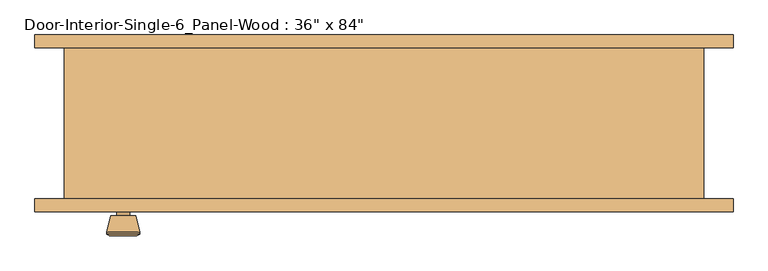
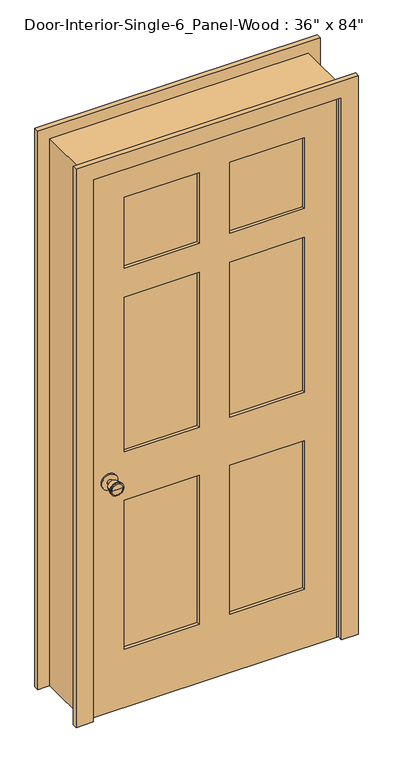
"""IFC4 building model written with IfcOpenShell, lengths in millimetres: door geometry."""

from ifc_helpers import new_model, si_unit, point, frame, frame_2d, origin, place, context, project, spatial, polyline, circle_curve, trimmed, segment, composite_curve, outline, extrude, faceted_brep, source, transform, mapped, element, save
from ifc_brep_helpers import plane_surface, cylinder_surface, revolved_surface, advanced_brep


def door_c5239341(model_context):
    return source(origin(), model_context, "Body", "SolidModel", [
        advanced_brep(
        [(-393.7, -70.2, 914.4), (-403.7, -70.2, 914.4), (-383.7, -70.2, 914.4), (-373.2241324, -21.2, 914.4), (-414.1758676, -21.2, 914.4), (-393.7, -21.2, 914.4), (-368.7, -23.0278681, 914.4), (-418.7, -23.0278681, 914.4), (-368.7, -26.4915463, 914.4), (-418.7, -26.4915463, 914.4), (-375.063764, -51.2, 914.4), (-412.336236, -51.2, 914.4), (-383.7, -51.2, 914.4), (-403.7, -51.2, 914.4)],
        [
            (0, 1),
            (1, 2, circle_curve(frame((-393.7, -70.2, 914.4), z_axis=(0.0, -1.0, 0.0), x_axis=(-1.0, 0.0, 0.0)), 10.0)),
            (2, 0),
            (2, 1, circle_curve(frame((-393.7, -70.2, 914.4), z_axis=(0.0, -1.0, 0.0), x_axis=(-1.0, 0.0, 0.0)), 10.0)),
            (3, 4, circle_curve(frame((-393.7, -21.2, 914.4), z_axis=(0.0, 1.0, 0.0), x_axis=(-1.0, 0.0, 0.0)), 20.4758676)),
            (4, 5),
            (5, 3),
            (4, 3, circle_curve(frame((-393.7, -21.2, 914.4), z_axis=(0.0, 1.0, 0.0), x_axis=(-1.0, 0.0, 0.0)), 20.4758676)),
            (6, 7, circle_curve(frame((-393.7, -23.0278681, 914.4), z_axis=(0.0, 1.0, 0.0), x_axis=(-1.0, 0.0, 0.0)), 25.0)),
            (7, 4),
            (3, 6),
            (7, 6, circle_curve(frame((-393.7, -23.0278681, 914.4), z_axis=(0.0, 1.0, 0.0), x_axis=(-1.0, 0.0, 0.0)), 25.0)),
            (8, 9, circle_curve(frame((-393.7, -26.4915463, 914.4), z_axis=(0.0, 1.0, 0.0), x_axis=(-1.0, 0.0, 0.0)), 25.0)),
            (9, 7),
            (6, 8),
            (9, 8, circle_curve(frame((-393.7, -26.4915463, 914.4), z_axis=(0.0, 1.0, 0.0), x_axis=(-1.0, 0.0, 0.0)), 25.0)),
            (10, 11, circle_curve(frame((-393.7, -51.2, 914.4), z_axis=(0.0, 1.0, 0.0), x_axis=(-1.0, 0.0, 0.0)), 18.636236)),
            (11, 9),
            (8, 10),
            (11, 10, circle_curve(frame((-393.7, -51.2, 914.4), z_axis=(0.0, 1.0, 0.0), x_axis=(-1.0, 0.0, 0.0)), 18.636236)),
            (12, 13, circle_curve(frame((-393.7, -51.2, 914.4), z_axis=(0.0, 1.0, 0.0), x_axis=(-1.0, 0.0, 0.0)), 10.0)),
            (13, 11),
            (10, 12),
            (13, 12, circle_curve(frame((-393.7, -51.2, 914.4), z_axis=(0.0, 1.0, 0.0), x_axis=(-1.0, 0.0, 0.0)), 10.0)),
            (1, 13),
            (12, 2),
        ],
        [
            plane_surface(frame((-393.7, -70.2, 914.4), z_axis=(0.0, -1.0, 0.0), x_axis=(-1.0, 0.0, 0.0))),
            plane_surface(frame((-393.7, -21.2, 914.4), z_axis=(0.0, 1.0, 0.0), x_axis=(-1.0, 0.0, 0.0))),
            revolved_surface(polyline([(-414.1758676, -21.2, 914.4), (-418.7, -23.0278681, 914.4)]), (-393.7, -70.2, 914.4), (0.0, -1.0, 0.0)),
            cylinder_surface(frame((-393.7, -70.2, 914.4), z_axis=(0.0, -1.0, 0.0), x_axis=(-1.0, 0.0, 0.0)), 25.0),
            revolved_surface(polyline([(-418.7, -26.4915463, 914.4), (-412.336236, -51.2, 914.4)]), (-393.7, -70.2, 914.4), (0.0, -1.0, 0.0)),
            plane_surface(frame((-393.7, -51.2, 914.4), z_axis=(0.0, -1.0, 0.0), x_axis=(-1.0, 0.0, 0.0))),
            cylinder_surface(frame((-393.7, -70.2, 914.4), z_axis=(0.0, -1.0, 0.0), x_axis=(-1.0, 0.0, 0.0)), 10.0),
        ],
        [
            (0, [[1, 2, 3]]),
            (0, [[-3, 4, -1]]),
            (1, [[5, 6, 7]]),
            (1, [[8, -7, -6]]),
            (2, [[9, 10, -5, 11]]),
            (2, [[12, -11, -8, -10]]),
            (3, [[13, 14, -9, 15]]),
            (3, [[16, -15, -12, -14]]),
            (4, [[17, 18, -13, 19]]),
            (4, [[20, -19, -16, -18]]),
            (5, [[21, 22, -17, 23]]),
            (5, [[24, -23, -20, -22]]),
            (6, [[-2, 25, -21, 26]]),
            (6, [[-4, -26, -24, -25]]),
        ],
    ),
        extrude(outline(composite_curve([segment(trimmed(circle_curve(frame_2d((914.4, -393.7)), 30.0), [point((914.4, -423.7))], [point((914.4, -363.7))], False, "CARTESIAN"), True, "CONTINUOUS"), segment(trimmed(circle_curve(frame_2d((914.4, -393.7)), 30.0), [point((914.4, -363.7))], [point((914.4, -423.7))], False, "CARTESIAN"), True, "CONTINUOUS")], self_intersect=False)), frame((0.0, -76.2, 0.0), z_axis=(0.0, 1.0, 0.0), x_axis=(0.0, 0.0, 1.0)), (0.0, 0.0, 1.0), 6.0),
        advanced_brep(
        [(-393.7, -117.125, 914.4), (-383.7, -117.125, 914.4), (-403.7, -117.125, 914.4), (-373.2241324, -166.125, 914.4), (-393.7, -166.125, 914.4), (-414.1758676, -166.125, 914.4), (-368.7, -164.2971319, 914.4), (-418.7, -164.2971319, 914.4), (-368.7, -160.8334537, 914.4), (-418.7, -160.8334537, 914.4), (-375.063764, -136.125, 914.4), (-412.336236, -136.125, 914.4), (-383.7, -136.125, 914.4), (-403.7, -136.125, 914.4)],
        [
            (0, 1),
            (1, 2, circle_curve(frame((-393.7, -117.125, 914.4), z_axis=(0.0, 1.0, 0.0), x_axis=(-1.0, 0.0, 0.0)), 10.0)),
            (2, 0),
            (2, 1, circle_curve(frame((-393.7, -117.125, 914.4), z_axis=(0.0, 1.0, 0.0), x_axis=(-1.0, 0.0, 0.0)), 10.0)),
            (3, 4),
            (4, 5),
            (5, 3, circle_curve(frame((-393.7, -166.125, 914.4), z_axis=(0.0, -1.0, 0.0), x_axis=(-1.0, 0.0, 0.0)), 20.4758676)),
            (3, 5, circle_curve(frame((-393.7, -166.125, 914.4), z_axis=(0.0, -1.0, 0.0), x_axis=(-1.0, 0.0, 0.0)), 20.4758676)),
            (6, 3),
            (5, 7),
            (7, 6, circle_curve(frame((-393.7, -164.2971319, 914.4), z_axis=(0.0, -1.0, 0.0), x_axis=(-1.0, 0.0, 0.0)), 25.0)),
            (6, 7, circle_curve(frame((-393.7, -164.2971319, 914.4), z_axis=(0.0, -1.0, 0.0), x_axis=(-1.0, 0.0, 0.0)), 25.0)),
            (8, 6),
            (7, 9),
            (9, 8, circle_curve(frame((-393.7, -160.8334537, 914.4), z_axis=(0.0, -1.0, 0.0), x_axis=(-1.0, 0.0, 0.0)), 25.0)),
            (8, 9, circle_curve(frame((-393.7, -160.8334537, 914.4), z_axis=(0.0, -1.0, 0.0), x_axis=(-1.0, 0.0, 0.0)), 25.0)),
            (10, 8),
            (9, 11),
            (11, 10, circle_curve(frame((-393.7, -136.125, 914.4), z_axis=(0.0, -1.0, 0.0), x_axis=(-1.0, 0.0, 0.0)), 18.636236)),
            (10, 11, circle_curve(frame((-393.7, -136.125, 914.4), z_axis=(0.0, -1.0, 0.0), x_axis=(-1.0, 0.0, 0.0)), 18.636236)),
            (12, 10),
            (11, 13),
            (13, 12, circle_curve(frame((-393.7, -136.125, 914.4), z_axis=(0.0, -1.0, 0.0), x_axis=(-1.0, 0.0, 0.0)), 10.0)),
            (12, 13, circle_curve(frame((-393.7, -136.125, 914.4), z_axis=(0.0, -1.0, 0.0), x_axis=(-1.0, 0.0, 0.0)), 10.0)),
            (1, 12),
            (13, 2),
        ],
        [
            plane_surface(frame((-393.7, -117.125, 914.4), z_axis=(0.0, 1.0, 0.0), x_axis=(-1.0, 0.0, 0.0))),
            plane_surface(frame((-393.7, -166.125, 914.4), z_axis=(0.0, -1.0, 0.0), x_axis=(-1.0, 0.0, 0.0))),
            revolved_surface(polyline([(-414.1758676, -166.125, 914.4), (-418.7, -164.2971319, 914.4)]), (-393.7, -117.125, 914.4), (0.0, 1.0, 0.0)),
            cylinder_surface(frame((-393.7, -117.125, 914.4), z_axis=(0.0, 1.0, 0.0), x_axis=(-1.0, 0.0, 0.0)), 25.0),
            revolved_surface(polyline([(-418.7, -160.8334537, 914.4), (-412.336236, -136.125, 914.4)]), (-393.7, -117.125, 914.4), (0.0, 1.0, 0.0)),
            plane_surface(frame((-393.7, -136.125, 914.4), z_axis=(0.0, 1.0, 0.0), x_axis=(-1.0, 0.0, 0.0))),
            cylinder_surface(frame((-393.7, -117.125, 914.4), z_axis=(0.0, 1.0, 0.0), x_axis=(-1.0, 0.0, 0.0)), 10.0),
        ],
        [
            (0, [[1, 2, 3]]),
            (0, [[-3, 4, -1]]),
            (1, [[5, 6, 7]]),
            (1, [[-6, -5, 8]]),
            (2, [[9, -7, 10, 11]]),
            (2, [[-10, -8, -9, 12]]),
            (3, [[13, -11, 14, 15]]),
            (3, [[-14, -12, -13, 16]]),
            (4, [[17, -15, 18, 19]]),
            (4, [[-18, -16, -17, 20]]),
            (5, [[21, -19, 22, 23]]),
            (5, [[-22, -20, -21, 24]]),
            (6, [[25, -23, 26, -2]]),
            (6, [[-26, -24, -25, -4]]),
        ],
    ),
        extrude(outline(composite_curve([segment(trimmed(circle_curve(frame_2d((914.4, -393.7)), 30.0), [point((914.4, -423.7))], [point((914.4, -363.7))], False, "CARTESIAN"), True, "CONTINUOUS"), segment(trimmed(circle_curve(frame_2d((914.4, -393.7)), 30.0), [point((914.4, -363.7))], [point((914.4, -423.7))], False, "CARTESIAN"), True, "CONTINUOUS")], self_intersect=False)), frame((0.0, -117.125, 0.0), z_axis=(0.0, 1.0, 0.0), x_axis=(0.0, 0.0, 1.0)), (0.0, 0.0, 1.0), 6.0),
        faceted_brep([(482.6, -111.125, 0.0), (457.2, -111.125, 0.0), (457.2, -76.2, 0.0), (444.5, -76.2, 0.0), (444.5, -41.275, 0.0), (457.2, -41.275, 0.0), (457.2, 117.475, 0.0), (482.6, 117.475, 0.0), (482.6, 117.475, 2159.0), (482.6, -111.125, 2159.0), (457.2, 117.475, 2133.6), (-457.2, 117.475, 2133.6), (-457.2, 117.475, 0.0), (-482.6, 117.475, 0.0), (-482.6, 117.475, 2159.0), (457.2, -41.275, 2133.6), (444.5, -41.275, 2120.9), (-444.5, -41.275, 2120.9), (-444.5, -41.275, 0.0), (-457.2, -41.275, 0.0), (-457.2, -41.275, 2133.6), (444.5, -76.2, 2120.9), (457.2, -76.2, 2133.6), (-457.2, -76.2, 2133.6), (-457.2, -76.2, 0.0), (-444.5, -76.2, 0.0), (-444.5, -76.2, 2120.9), (457.2, -111.125, 2133.6), (-482.6, -111.125, 2159.0), (-482.6, -111.125, 0.0), (-457.2, -111.125, 0.0), (-457.2, -111.125, 2133.6)], [[[0, 1, 2, 3, 4, 5, 6, 7]], [[7, 8, 9, 0]], [[6, 10, 11, 12, 13, 14, 8, 7]], [[5, 15, 10, 6]], [[4, 16, 17, 18, 19, 20, 15, 5]], [[3, 21, 16, 4]], [[2, 22, 23, 24, 25, 26, 21, 3]], [[1, 27, 22, 2]], [[0, 9, 28, 29, 30, 31, 27, 1]], [[8, 14, 28, 9]], [[15, 20, 11, 10]], [[21, 26, 17, 16]], [[27, 31, 23, 22]], [[29, 13, 12, 19, 18, 25, 24, 30]], [[14, 13, 29, 28]], [[20, 19, 12, 11]], [[26, 25, 18, 17]], [[31, 30, 24, 23]]]),
        extrude(outline(polyline([(2133.6, -457.2), (0.0, -457.2), (0.0, 457.2), (2133.6, 457.2), (2133.6, -457.2)]), holes=[polyline([(2014.5375, 57.15), (2014.5375, 336.55), (1735.1375, 336.55), (1735.1375, 57.15), (2014.5375, 57.15)]), polyline([(1620.8375, 336.55), (1009.65, 336.55), (1009.65, 57.15), (1620.8375, 57.15), (1620.8375, 336.55)]), polyline([(1009.65, -57.15), (1009.65, -336.55), (1620.8375, -336.55), (1620.8375, -57.15), (1009.65, -57.15)]), polyline([(1735.1375, -336.55), (2014.5375, -336.55), (2014.5375, -57.15), (1735.1375, -57.15), (1735.1375, -336.55)]), polyline([(819.15, 57.15), (819.15, 336.55), (231.775, 336.55), (231.775, 57.15), (819.15, 57.15)]), polyline([(231.775, -57.15), (231.775, -336.55), (819.15, -336.55), (819.15, -57.15), (231.775, -57.15)])]), frame((0.0, -111.125, 0.0), z_axis=(0.0, 1.0, 0.0), x_axis=(0.0, 0.0, 1.0)), (0.0, 0.0, 1.0), 34.925),
        extrude(outline(polyline([(336.55, -87.8416667), (336.55, -99.4833333), (57.15, -99.4833333), (57.15, -87.8416667), (336.55, -87.8416667)])), frame((0.0, 0.0, 1735.1375), z_axis=(0.0, 0.0, 1.0), x_axis=(1.0, 0.0, 0.0)), (0.0, 0.0, 1.0), 279.4),
        extrude(outline(polyline([(336.55, -87.8416667), (336.55, -99.4833333), (57.15, -99.4833333), (57.15, -87.8416667), (336.55, -87.8416667)])), frame((0.0, 0.0, 1009.65), z_axis=(0.0, 0.0, 1.0), x_axis=(1.0, 0.0, 0.0)), (0.0, 0.0, 1.0), 611.1875),
        extrude(outline(polyline([(-57.15, -87.8416667), (-57.15, -99.4833333), (-336.55, -99.4833333), (-336.55, -87.8416667), (-57.15, -87.8416667)])), frame((0.0, 0.0, 1009.65), z_axis=(0.0, 0.0, 1.0), x_axis=(1.0, 0.0, 0.0)), (0.0, 0.0, 1.0), 611.1875),
        extrude(outline(polyline([(-57.15, -87.8416667), (-57.15, -99.4833333), (-336.55, -99.4833333), (-336.55, -87.8416667), (-57.15, -87.8416667)])), frame((0.0, 0.0, 1735.1375), z_axis=(0.0, 0.0, 1.0), x_axis=(1.0, 0.0, 0.0)), (0.0, 0.0, 1.0), 279.4),
        extrude(outline(polyline([(336.55, -87.8416667), (336.55, -99.4833333), (57.15, -99.4833333), (57.15, -87.8416667), (336.55, -87.8416667)])), frame((0.0, 0.0, 231.775), z_axis=(0.0, 0.0, 1.0), x_axis=(1.0, 0.0, 0.0)), (0.0, 0.0, 1.0), 587.375),
        extrude(outline(polyline([(-57.15, -87.8416667), (-57.15, -99.4833333), (-336.55, -99.4833333), (-336.55, -87.8416667), (-57.15, -87.8416667)])), frame((0.0, 0.0, 231.775), z_axis=(0.0, 0.0, 1.0), x_axis=(1.0, 0.0, 0.0)), (0.0, 0.0, 1.0), 587.375),
        extrude(outline(polyline([(0.0, 527.05), (2203.45, 527.05), (2203.45, -527.05), (0.0, -527.05), (0.0, -463.55), (2139.95, -463.55), (2139.95, 463.55), (0.0, 463.55), (0.0, 527.05)])), frame((0.0, -130.175, 0.0), z_axis=(0.0, 1.0, 0.0), x_axis=(0.0, 0.0, 1.0)), (0.0, 0.0, 1.0), 19.05),
        extrude(outline(polyline([(0.0, 527.05), (2203.45, 527.05), (2203.45, -527.05), (0.0, -527.05), (0.0, -463.55), (2139.95, -463.55), (2139.95, 463.55), (0.0, 463.55), (0.0, 527.05)])), frame((0.0, 117.475, 0.0), z_axis=(0.0, 1.0, 0.0), x_axis=(0.0, 0.0, 1.0)), (0.0, 0.0, 1.0), 19.05),
    ])


if __name__ == "__main__":
    model = new_model("IFC4")
    model_context = context("Model", 3, world=origin())
    ifc_project = project(units=[si_unit("LENGTHUNIT", "METRE", prefix="MILLI")], contexts=[model_context])
    site = spatial("IfcSite", under=ifc_project)
    building = spatial("IfcBuilding", under=site)
    placement = place(None, origin())
    door_shape = door_c5239341(model_context)
    element("IfcDoor", 1, ObjectType="Door-Interior-Single-6_Panel-Wood : 36\" x 84\"", at=placement, inside=building, context=model_context, shape_type="MappedRepresentation", body=[
        mapped(door_shape, transform((0.0, 0.0, 0.0), x_axis=(1.0, 0.0, 0.0), y_axis=(0.0, 1.0, 0.0), z_axis=(0.0, 0.0, 1.0))),
    ])
    save(model, "model.ifc")

# Revit data of these elements
# Type "Door-Interior-Single-6_Panel-Wood : 36\" x 84\""
#   Type Mark = "9"
#   Assembly Code = "C1020300"
#   Analytic Construction = "Wooden"
#   Top Rail = 0' - 4 11/16"
#   Top Panel = 0' - 11"
#   Thickness = 0' - 1 3/8"
#   Thermal Resistance (R) = 2.5876 (h·ft²·°F)/BTU
#   Swing Angle [instance default] = 90.00°
#   Stiles = 0' - 4 3/4"
#   Rough Width = 3' - 2"
#   Rough Height = 7' - 1"
#   Mullion = 0' - 4 1/2"
#   Lock Rail = 0' - 7 1/2"
#   Intermediate Rail = 0' - 4 1/2"
#   Height = 7' - 0"
#   Width = 3' - 0"
#   Heat Transfer Coefficient (U) = 0.3865 BTU/(h·ft²·°F)
#   Bottom Rail = 0' - 9 1/8"
#   Trim Material = Cherry
#   Panel Material = Cherry
#   Frame Material = Cherry
#   Door Handle Material = Aluminum
#   Visual Light Transmittance = 0
#   Solar Heat Gain Coefficient = 0
#   Wall Closure = (empty or 0)
#   Function = (empty or 0)
# Element 1 (IfcDoor, "Door-Interior-Single-6_Panel-Wood : 36\" x 84\"")
#   Materials on its faces: "Cherry", "Aluminum"
# Materials
#   "Cherry": class "Wood", colour RGB 226 177 128, transparency 0, Description = "Prunus Serotina", Cost = 0
#   "Aluminum": class "Metal", colour RGB 247 247 247, transparency 0, Description = "Aluminum 6061", Cost = 0
